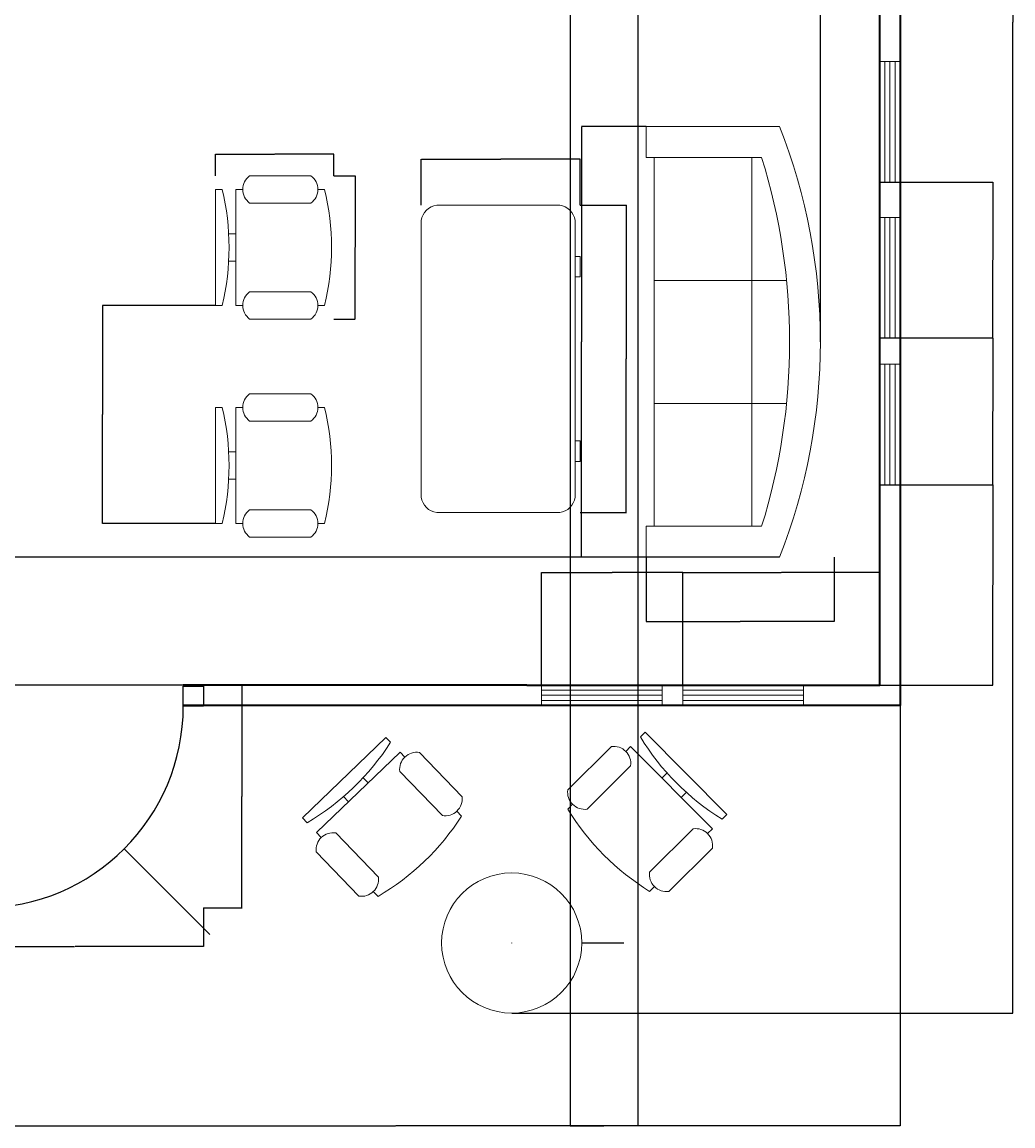
# Model space of a CAD drawing. Units: millimetres. Extents: x 1312 to 12932, y -881 to 10062.
# Tile 3 of 4: x 8020 to 12932, y -881 to 4591. Entities that reach past the tile are written whole.
import ezdxf

# ---------------------------------------------------------------- set-up
doc = ezdxf.new("R2010")
doc.units = ezdxf.units.MM
for name, color, linetype, lineweight in [('A-ANNO-DIMS', 2, 'Continuous', 18), ('A-DOOR', 3, 'Continuous', 25), ('A-FURN', 8, 'Continuous', 18), ('A-GLAZ', 4, 'Continuous', 18), ('A-WALL', 7, 'Continuous', 35)]:
    doc.layers.add(name, color=color, linetype=linetype, lineweight=lineweight)
doc.styles.get("Standard").update_dxf_attribs({"font": 'arial.ttf'})
doc.dimstyles.get("Standard").update_dxf_attribs({"dimtxt": 0.18, "dimasz": 0.18, "dimexe": 0.18, "dimexo": 0.0625, "dimgap": 0.09, "dimtad": 0, "dimtih": 1, "dimtoh": 1, "dimdec": 4, "dimzin": 0, "dimdsep": 46, "dimtxsty": 'Standard', "dimcen": 0.09, "dimadec": 0, "dimazin": 0, "dimtfac": 1, "dimtdec": 4, "dimtofl": 0, "dimtmove": 0, "dimatfit": 3, "dimfxl": 1, "dimtolj": 1, "dimtzin": 0, "dimarcsym": 0})

# ---------------------------------------------------------------- blocks, each defined once
blk = doc.blocks.new('Sofa - Roundback 7 ft.')
for p, q in [((-12.00002, -32.4421), (-12.00003, -6.5971)), ((11.99997, -32.4421), (11.99998, -6.5971)), ((-36.000027, -34), (-36.000027, -11.4696)), ((35.99998, -34), (35.99998, -11.4696)), ((-35.999844, -13.3819), (35.9998, -13.3819)), ((-36.000027, -32.4421), (35.99998, -32.4421))]:
    blk.add_line(p, q)
for points in [[(-36.000027, -34), (-42.000027, -34), (-42.000027, -8)], [(41.99998, -8), (41.99998, -34), (35.99998, -34)]]:
    blk.add_lwpolyline(points)
for centre, radius, start, end in [((0, -114.25), 114.25, 68.43141, 111.5686), ((-0.00001, -127.1968), 121.1968, 72.72033, 107.2797)]:
    blk.add_arc(centre, radius, start, end)
blk = doc.blocks.new('Chair - Desk')
for p, q in [((-8.5, 0), (-8.5, -1)), ((-8.5, 0), (8.5, 0)), ((8.5, 0), (8.5, -1)), ((-8.5, -3), (-8.5, -4)), ((-8.5, -3), (8.5, -3)), ((-2, -3), (-2, -1.9355)), ((2, -1.9576), (2, -3)), ((8.5, -3), (8.5, -4)), ((-10.5, -5), (-10.5, -14)), ((-6.5, -14), (-6.5, -5)), ((6.5, -5), (6.5, -14)), ((10.5, -14), (10.5, -5)), ((-8.5, -15), (-8.5, -16)), ((8.5, -15), (8.5, -16))]:
    blk.add_line(p, q)
for centre, radius, start, end in [((0, 34.625), 36.625, 256.5803, 283.4197), ((-8.5, -6.5), 2.5, 36.8699, 143.1301), ((8.5, -6.5), 2.5, 36.8699, 143.1301), ((-8.5, -12.5), 2.5, 216.8699, 323.1301), ((8.5, -12.5), 2.5, 216.8699, 323.1301), ((0, 19.625), 36.625, 256.5803, 283.4197)]:
    blk.add_arc(centre, radius, start, end)
blk = doc.blocks.new('Desk - 30 x 60 in.')
for p, q in [((-26.999995, 0), (26.999995, 0)), ((-29.999995, -27), (-29.999995, -3)), ((29.999995, -3), (29.999995, -27)), ((26.999995, -30), (-26.999995, -30)), ((-20.000005, -30), (-20.000005, -31)), ((-16.000005, -31), (-16.000005, -30)), ((15.999995, -31), (15.999995, -30)), ((19.999995, -30), (19.999995, -31)), ((-20.000005, -31), (-16.000005, -31)), ((19.999995, -31), (15.999995, -31))]:
    blk.add_line(p, q)
for centre, start, end in [((-26.499995, -3.5), 98.1301, 171.8699), ((26.499995, -3.5), 8.130102, 81.8699), ((-26.499995, -26.5), 188.1301, 261.8699), ((26.499995, -26.5), 278.1301, 351.8699)]:
    blk.add_arc(centre, 3.535534, start, end)
blk = doc.blocks.new('Window - Wood Frame 36 in. Wide plan')
for p, q in [((0, 6), (0, 0)), ((0, 4.5), (36, 4.5)), ((36, 6), (36, 0)), ((0, 3), (36, 3)), ((0, 1.5), (36, 1.5))]:
    blk.add_line(p, q)
blk = doc.blocks.new('DOOR-SINGLE-1000')
for p, q in [((0, 1003.8), (0, 1103.8)), ((0, 1103.8), (100, 1103.8)), ((100, 1103.8), (100, 1003.8)), ((1174.2, 1000), (1174.2, 1100)), ((1174.2, 1100), (1274.2, 1100)), ((1274.2, 1100), (1274.2, 1000)), ((100, 1003.8), (0, 1003.8)), ((100, 1000), (174.2, 1000)), ((100, 0), (100, 1000)), ((174.2, 1000), (174.2, 0)), ((1274.2, 1000), (1174.2, 1000)), ((174.2, 0), (100, 0))]:
    blk.add_line(p, q)
blk.add_arc((174.2, 1000), 1000, 270, 0)
blk = doc.blocks.new('*D15')
at = {"layer": 'A-ANNO-DIMS', "color": 0, "lineweight": -2, "transparency": 16777216}
for p, q in [((7644.9, 199.3), (7644.9, 8)), ((8919.1, 199.3), (8919.1, 8)), ((7645.1, 8.2), (8280.6, 8.2)), ((8918.9, 8.2), (8283.4, 8.2))]:
    blk.add_line(p, q, dxfattribs=at)
at = {"layer": 'A-ANNO-DIMS', "color": 0, "transparency": 16777216}
for points in [[(7645.1, 8.2), (7645.1, 8.2), (7644.9, 8.2)], [(8918.9, 8.2), (8918.9, 8.2), (8919.1, 8.2)]]:
    blk.add_solid(points, dxfattribs=at)
at = {"layer": 'Defpoints', "color": 0, "transparency": 16777216}
for p in [(7644.9, 199.3), (8919.1, 199.3), (8919.1, 8.2)]:
    blk.add_point(p, dxfattribs=at)
at = {"layer": 'A-ANNO-DIMS', "color": 0, "transparency": 16777216, "insert": (8282, 8.2), "char_height": 0.18, "attachment_point": 5}
blk.add_mtext('\\A1;DOOR UNIT 1274 TYP.', dxfattribs=at)
blk = doc.blocks.new('*D16')
at = {"layer": 'A-ANNO-DIMS', "color": 0, "lineweight": -2, "transparency": 16777216}
for p, q in [((8919.2, 1303.1), (9110.4, 1303.1)), ((9110.2, 1302.9), (9110.2, 751.4)), ((9110.2, 199.5), (9110.2, 751)), ((8919.2, 199.3), (9110.4, 199.3))]:
    blk.add_line(p, q, dxfattribs=at)
at = {"layer": 'A-ANNO-DIMS', "color": 0, "transparency": 16777216}
for points in [[(9110.2, 1302.9), (9110.3, 1302.9), (9110.2, 1303.1)], [(9110.2, 199.5), (9110.3, 199.5), (9110.2, 199.3)]]:
    blk.add_solid(points, dxfattribs=at)
at = {"layer": 'Defpoints', "color": 0, "transparency": 16777216}
for p in [(8919.1, 1303.1), (9110.2, 1303.1), (8919.1, 199.3)]:
    blk.add_point(p, dxfattribs=at)
at = {"layer": 'A-ANNO-DIMS', "color": 0, "transparency": 16777216, "insert": (9110.2, 751.2), "char_height": 0.18, "attachment_point": 5}
blk.add_mtext('\\A1;1104 TYP.', dxfattribs=at)
blk = doc.blocks.new('*D17')
at = {"layer": 'A-ANNO-DIMS', "color": 0, "lineweight": -2, "transparency": 16777216}
for p, q in [((9564.9, 3829), (9671.6, 3829)), ((9671.4, 3828.8), (9671.4, 3474)), ((9671.4, 3118.8), (9671.4, 3473.6)), ((9564.9, 3118.7), (9671.6, 3118.7))]:
    blk.add_line(p, q, dxfattribs=at)
at = {"layer": 'A-ANNO-DIMS', "color": 0, "transparency": 16777216}
for points in [[(9671.4, 3828.8), (9671.4, 3828.8), (9671.4, 3829)], [(9671.4, 3118.8), (9671.4, 3118.8), (9671.4, 3118.7)]]:
    blk.add_solid(points, dxfattribs=at)
at = {"layer": 'Defpoints', "color": 0, "transparency": 16777216}
for p in [(9564.9, 3829), (9671.4, 3829), (9564.9, 3118.7)]:
    blk.add_point(p, dxfattribs=at)
at = {"layer": 'A-ANNO-DIMS', "color": 0, "transparency": 16777216, "insert": (9671.4, 3473.8), "char_height": 0.18, "attachment_point": 5}
blk.add_mtext('\\A1;CHAIR 710 TYP.', dxfattribs=at)
blk = doc.blocks.new('*D18')
at = {"layer": 'A-ANNO-DIMS', "color": 0, "lineweight": -2, "transparency": 16777216}
for p, q in [((8978.6, 3829), (8978.6, 3935.7)), ((8978.8, 3935.5), (9271.1, 3935.5)), ((9564.7, 3935.5), (9272.3, 3935.5)), ((9564.9, 3829), (9564.9, 3935.7))]:
    blk.add_line(p, q, dxfattribs=at)
at = {"layer": 'A-ANNO-DIMS', "color": 0, "transparency": 16777216}
for points in [[(8978.8, 3935.5), (8978.8, 3935.5), (8978.6, 3935.5)], [(9564.7, 3935.5), (9564.7, 3935.5), (9564.9, 3935.5)]]:
    blk.add_solid(points, dxfattribs=at)
at = {"layer": 'Defpoints', "color": 0, "transparency": 16777216}
for p in [(8978.6, 3935.5), (8978.6, 3829), (9564.9, 3829)]:
    blk.add_point(p, dxfattribs=at)
at = {"layer": 'A-ANNO-DIMS', "color": 0, "transparency": 16777216, "insert": (9271.7, 3935.5), "char_height": 0.18, "attachment_point": 5}
blk.add_mtext('\\A1;586 TYP.', dxfattribs=at)
blk = doc.blocks.new('*D37')
at = {"layer": 'A-ANNO-DIMS', "color": 0, "lineweight": -2, "transparency": 16777216}
for p, q in [((11113.5, 4072.2), (10793.4, 4072.2)), ((10793.6, 4072), (10793.6, 3005.6)), ((10793.6, 1938.8), (10793.6, 3005.2)), ((11113.5, 1938.6), (10793.4, 1938.6))]:
    blk.add_line(p, q, dxfattribs=at)
at = {"layer": 'A-ANNO-DIMS', "color": 0, "transparency": 16777216}
for points in [[(10793.5, 4072), (10793.6, 4072), (10793.6, 4072.2)], [(10793.5, 1938.8), (10793.6, 1938.8), (10793.6, 1938.6)]]:
    blk.add_solid(points, dxfattribs=at)
at = {"layer": 'Defpoints', "color": 0, "transparency": 16777216}
for p in [(11113.6, 4072.2), (10793.6, 1938.6), (11113.6, 1938.6)]:
    blk.add_point(p, dxfattribs=at)
at = {"layer": 'A-ANNO-DIMS', "color": 0, "transparency": 16777216, "insert": (10793.6, 3005.4), "char_height": 0.18, "attachment_point": 5}
blk.add_mtext('\\A1;SOFA 2134', dxfattribs=at)
blk = doc.blocks.new('*D38')
at = {"layer": 'A-ANNO-DIMS', "color": 0, "lineweight": -2, "transparency": 16777216}
for p, q in [((11113.6, 1938.5), (11113.6, 1618.4)), ((12044.9, 1938.5), (12044.9, 1618.4)), ((11113.8, 1618.6), (11579, 1618.6)), ((12044.8, 1618.6), (11579.6, 1618.6))]:
    blk.add_line(p, q, dxfattribs=at)
at = {"layer": 'A-ANNO-DIMS', "color": 0, "transparency": 16777216}
for points in [[(11113.8, 1618.6), (11113.8, 1618.5), (11113.6, 1618.6)], [(12044.8, 1618.6), (12044.8, 1618.5), (12044.9, 1618.6)]]:
    blk.add_solid(points, dxfattribs=at)
at = {"layer": 'Defpoints', "color": 0, "transparency": 16777216}
for p in [(11113.6, 1938.6), (12044.9, 1938.6), (12044.9, 1618.6)]:
    blk.add_point(p, dxfattribs=at)
at = {"layer": 'A-ANNO-DIMS', "color": 0, "transparency": 16777216, "insert": (11579.3, 1618.6), "char_height": 0.18, "attachment_point": 5}
blk.add_mtext('\\A1;931', dxfattribs=at)
blk = doc.blocks.new('*D39')
at = {"layer": 'A-ANNO-DIMS', "color": 0, "lineweight": -2, "transparency": 16777216}
for p, q in [((10786.6, 3683), (11015.3, 3683)), ((11015.1, 3682.9), (11015.1, 2921.2)), ((11015.1, 2159.2), (11015.1, 2920.9)), ((10786.6, 2159), (11015.3, 2159))]:
    blk.add_line(p, q, dxfattribs=at)
at = {"layer": 'A-ANNO-DIMS', "color": 0, "transparency": 16777216}
for points in [[(11015.1, 3682.9), (11015.1, 3682.9), (11015.1, 3683)], [(11015.1, 2159.2), (11015.1, 2159.2), (11015.1, 2159)]]:
    blk.add_solid(points, dxfattribs=at)
at = {"layer": 'Defpoints', "color": 0, "transparency": 16777216}
for p in [(10786.5, 3683), (11015.1, 3683), (10786.5, 2159)]:
    blk.add_point(p, dxfattribs=at)
at = {"layer": 'A-ANNO-DIMS', "color": 0, "transparency": 16777216, "insert": (11015.1, 2921), "char_height": 0.18, "attachment_point": 5}
blk.add_mtext('\\A1;DESK 1524', dxfattribs=at)
blk = doc.blocks.new('*D40')
at = {"layer": 'A-ANNO-DIMS', "color": 0, "lineweight": -2, "transparency": 16777216}
for p, q in [((9999.1, 3683.1), (9999.1, 3911.8)), ((9999.3, 3911.6), (10392.5, 3911.6)), ((10786.3, 3911.6), (10393.1, 3911.6)), ((10786.5, 3683.1), (10786.5, 3911.8))]:
    blk.add_line(p, q, dxfattribs=at)
at = {"layer": 'A-ANNO-DIMS', "color": 0, "transparency": 16777216}
for points in [[(9999.3, 3911.7), (9999.3, 3911.6), (9999.1, 3911.6)], [(10786.3, 3911.7), (10786.3, 3911.6), (10786.5, 3911.6)]]:
    blk.add_solid(points, dxfattribs=at)
at = {"layer": 'Defpoints', "color": 0, "transparency": 16777216}
for p in [(9999.1, 3911.6), (9999.1, 3683), (10786.5, 3683)]:
    blk.add_point(p, dxfattribs=at)
at = {"layer": 'A-ANNO-DIMS', "color": 0, "transparency": 16777216, "insert": (10392.8, 3911.6), "char_height": 0.18, "attachment_point": 5}
blk.add_mtext('\\A1;787', dxfattribs=at)
blk = doc.blocks.new('*D59')
at = {"layer": 'A-ANNO-DIMS', "color": 0, "lineweight": -2, "transparency": 16777216}
for p, q in [((7372, 1203), (7372, -881.3)), ((12372, 1203), (12372, -881.3)), ((7372.2, -881.1), (9871.6, -881.1)), ((12371.8, -881.1), (9872.4, -881.1))]:
    blk.add_line(p, q, dxfattribs=at)
at = {"layer": 'A-ANNO-DIMS', "color": 0, "transparency": 16777216}
for points in [[(7372.2, -881), (7372.2, -881.1), (7372, -881.1)], [(12371.8, -881), (12371.8, -881.1), (12372, -881.1)]]:
    blk.add_solid(points, dxfattribs=at)
at = {"layer": 'Defpoints', "color": 0, "transparency": 16777216}
for p in [(7372, 1203.1), (12372, 1203.1), (12372, -881.1)]:
    blk.add_point(p, dxfattribs=at)
at = {"layer": 'A-ANNO-DIMS', "color": 0, "transparency": 16777216, "insert": (9872, -881.1), "char_height": 0.18, "attachment_point": 5}
blk.add_mtext('\\A1;5000', dxfattribs=at)
blk = doc.blocks.new('*D72')
at = {"layer": 'A-ANNO-DIMS', "color": 0, "lineweight": -2, "transparency": 16777216}
for p, q in [((10594.2, 1303.2), (10594.2, 1862.5)), ((10594.4, 1862.3), (10944.4, 1862.3)), ((11295.1, 1862.3), (10945.1, 1862.3)), ((11295.3, 1303.2), (11295.3, 1862.5))]:
    blk.add_line(p, q, dxfattribs=at)
at = {"layer": 'A-ANNO-DIMS', "color": 0, "transparency": 16777216}
for points in [[(10594.4, 1862.4), (10594.4, 1862.3), (10594.2, 1862.3)], [(11295.1, 1862.4), (11295.1, 1862.3), (11295.3, 1862.3)]]:
    blk.add_solid(points, dxfattribs=at)
at = {"layer": 'Defpoints', "color": 0, "transparency": 16777216}
for p in [(11295.3, 1862.3), (10594.2, 1303.1), (11295.3, 1303.1)]:
    blk.add_point(p, dxfattribs=at)
at = {"layer": 'A-ANNO-DIMS', "color": 0, "transparency": 16777216, "insert": (10944.8, 1862.3), "char_height": 0.18, "attachment_point": 5}
blk.add_mtext('\\A1;701.1', dxfattribs=at)
blk = doc.blocks.new('*D73')
at = {"layer": 'A-ANNO-DIMS', "color": 0, "lineweight": -2, "transparency": 16777216}
for p, q in [((11295.3, 1303.2), (11295.3, 1862.5)), ((11295.5, 1862.3), (11783.3, 1862.3)), ((12271.8, 1862.3), (11784, 1862.3)), ((12272, 1303.2), (12272, 1862.5))]:
    blk.add_line(p, q, dxfattribs=at)
at = {"layer": 'A-ANNO-DIMS', "color": 0, "transparency": 16777216}
for points in [[(11295.5, 1862.4), (11295.5, 1862.3), (11295.3, 1862.3)], [(12271.8, 1862.4), (12271.8, 1862.3), (12272, 1862.3)]]:
    blk.add_solid(points, dxfattribs=at)
at = {"layer": 'Defpoints', "color": 0, "transparency": 16777216}
for p in [(12272, 1862.3), (11295.3, 1303.1), (12272, 1303.1)]:
    blk.add_point(p, dxfattribs=at)
at = {"layer": 'A-ANNO-DIMS', "color": 0, "transparency": 16777216, "insert": (11783.6, 1862.3), "char_height": 0.18, "attachment_point": 5}
blk.add_mtext('\\A1;976.7', dxfattribs=at)
blk = doc.blocks.new('*D74')
at = {"layer": 'A-ANNO-DIMS', "color": 0, "lineweight": -2, "transparency": 16777216}
for p, q in [((12272.4, 2297.2), (12831.7, 2297.1)), ((12831.6, 2296.9), (12831.4, 1800.2)), ((12831.2, 1303.1), (12831.4, 1799.8)), ((12272.1, 1303.1), (12831.4, 1302.9))]:
    blk.add_line(p, q, dxfattribs=at)
at = {"layer": 'A-ANNO-DIMS', "color": 0, "transparency": 16777216}
for points in [[(12831.5, 2296.9), (12831.6, 2296.9), (12831.6, 2297.1)], [(12831.2, 1303.1), (12831.3, 1303.1), (12831.2, 1302.9)]]:
    blk.add_solid(points, dxfattribs=at)
at = {"layer": 'Defpoints', "color": 0, "transparency": 16777216}
for p in [(12272.3, 2297.2), (12272, 1303.1), (12831.2, 1302.9)]:
    blk.add_point(p, dxfattribs=at)
at = {"layer": 'A-ANNO-DIMS', "color": 0, "transparency": 16777216, "insert": (12831.4, 1800), "char_height": 0.18, "attachment_point": 5}
blk.add_mtext('\\A1;994.1', dxfattribs=at)
blk = doc.blocks.new('*D75')
at = {"layer": 'A-ANNO-DIMS', "color": 0, "lineweight": -2, "transparency": 16777216}
for p, q in [((12272.4, 3024.6), (12831.7, 3024.6)), ((12831.6, 3024.4), (12831.6, 2661.1)), ((12831.6, 2297.4), (12831.6, 2660.7)), ((12272.4, 2297.2), (12831.7, 2297.2))]:
    blk.add_line(p, q, dxfattribs=at)
at = {"layer": 'A-ANNO-DIMS', "color": 0, "transparency": 16777216}
for points in [[(12831.5, 3024.4), (12831.6, 3024.4), (12831.6, 3024.6)], [(12831.5, 2297.4), (12831.6, 2297.4), (12831.6, 2297.2)]]:
    blk.add_solid(points, dxfattribs=at)
at = {"layer": 'Defpoints', "color": 0, "transparency": 16777216}
for p in [(12272.3, 3024.6), (12272.3, 2297.2), (12831.6, 2297.2)]:
    blk.add_point(p, dxfattribs=at)
at = {"layer": 'A-ANNO-DIMS', "color": 0, "transparency": 16777216, "insert": (12831.6, 2660.9), "char_height": 0.18, "attachment_point": 5}
blk.add_mtext('\\A1;727.4', dxfattribs=at)
blk = doc.blocks.new('*D76')
at = {"layer": 'A-ANNO-DIMS', "color": 0, "lineweight": -2, "transparency": 16777216}
for p, q in [((12272.4, 3797.7), (12831.7, 3797.7)), ((12831.6, 3797.5), (12831.6, 3411.3)), ((12831.6, 3024.8), (12831.6, 3411)), ((12272.4, 3024.6), (12831.7, 3024.6))]:
    blk.add_line(p, q, dxfattribs=at)
at = {"layer": 'A-ANNO-DIMS', "color": 0, "transparency": 16777216}
for points in [[(12831.5, 3797.5), (12831.6, 3797.5), (12831.6, 3797.7)], [(12831.5, 3024.8), (12831.6, 3024.8), (12831.6, 3024.6)]]:
    blk.add_solid(points, dxfattribs=at)
at = {"layer": 'Defpoints', "color": 0, "transparency": 16777216}
for p in [(12272.3, 3797.7), (12272.3, 3024.6), (12831.6, 3024.6)]:
    blk.add_point(p, dxfattribs=at)
at = {"layer": 'A-ANNO-DIMS', "color": 0, "transparency": 16777216, "insert": (12831.6, 3411.1), "char_height": 0.18, "attachment_point": 5}
blk.add_mtext('\\A1;773', dxfattribs=at)
blk = doc.blocks.new('*D81')
at = {"layer": 'A-ANNO-DIMS', "color": 0, "lineweight": -2, "transparency": 16777216}
for p, q in [((12372.1, 9503.1), (12931.4, 9503.1)), ((12931.2, 9502.9), (12931.2, 4590.8)), ((12931.2, -321.6), (12931.2, 4590.4)), ((10447.2, -321.8), (12931.4, -321.8))]:
    blk.add_line(p, q, dxfattribs=at)
at = {"layer": 'A-ANNO-DIMS', "color": 0, "transparency": 16777216}
for points in [[(12931.2, 9502.9), (12931.3, 9502.9), (12931.2, 9503.1)], [(12931.2, -321.6), (12931.3, -321.6), (12931.2, -321.8)]]:
    blk.add_solid(points, dxfattribs=at)
at = {"layer": 'Defpoints', "color": 0, "transparency": 16777216}
for p in [(12372, 9503.1), (12931.2, 9503.1), (10447.2, -321.8)]:
    blk.add_point(p, dxfattribs=at)
at = {"layer": 'A-ANNO-DIMS', "color": 0, "transparency": 16777216, "insert": (12931.2, 4590.6), "char_height": 0.18, "attachment_point": 5}
blk.add_mtext('\\A1;9825', dxfattribs=at)
blk = doc.blocks.new('*D90')
at = {"layer": 'A-ANNO-DIMS', "color": 0, "lineweight": -2, "transparency": 16777216}
for p, q in [((10737.2, 9364.9), (10737.2, -881.3)), ((11072, 9403), (11072, -881.3)), ((10737.4, -881.1), (10904.2, -881.1)), ((11071.8, -881.1), (10905, -881.1))]:
    blk.add_line(p, q, dxfattribs=at)
at = {"layer": 'A-ANNO-DIMS', "color": 0, "transparency": 16777216}
for points in [[(10737.4, -881), (10737.4, -881.1), (10737.2, -881.1)], [(11071.8, -881), (11071.8, -881.1), (11072, -881.1)]]:
    blk.add_solid(points, dxfattribs=at)
at = {"layer": 'Defpoints', "color": 0, "transparency": 16777216}
for p in [(10737.2, 9365), (11072, 9403.1), (11072, -881.1)]:
    blk.add_point(p, dxfattribs=at)
at = {"layer": 'A-ANNO-DIMS', "color": 0, "transparency": 16777216, "insert": (10904.6, -881.1), "char_height": 0.18, "attachment_point": 5}
blk.add_mtext('\\A1;334.8', dxfattribs=at)
blk = doc.blocks.new('*D95')
at = {"layer": 'A-ANNO-DIMS', "color": 0, "lineweight": -2, "transparency": 16777216}
for p, q in [((11977.2, 3005.5), (11977.2, 10062.5)), ((11977.4, 10062.3), (12124.4, 10062.3)), ((12272.1, 10062.3), (12125.1, 10062.3)), ((12272.3, 3024.7), (12272.3, 10062.5))]:
    blk.add_line(p, q, dxfattribs=at)
at = {"layer": 'A-ANNO-DIMS', "color": 0, "transparency": 16777216}
for points in [[(11977.4, 10062.3), (11977.4, 10062.3), (11977.2, 10062.3)], [(12272.1, 10062.3), (12272.1, 10062.3), (12272.3, 10062.3)]]:
    blk.add_solid(points, dxfattribs=at)
at = {"layer": 'Defpoints', "color": 0, "transparency": 16777216}
for p in [(12272.3, 10062.3), (12272.3, 3024.6), (11977.2, 3005.4)]:
    blk.add_point(p, dxfattribs=at)
at = {"layer": 'A-ANNO-DIMS', "color": 0, "transparency": 16777216, "insert": (12124.8, 10062.3), "char_height": 0.18, "attachment_point": 5}
blk.add_mtext('\\A1;295.1', dxfattribs=at)
blk = doc.blocks.new('*D96')
at = {"layer": 'A-ANNO-DIMS', "color": 0, "lineweight": -2, "transparency": 16777216}
for p, q in [((11773.9, 1938.6), (1312.6, 1938.6)), ((1312.7, 1938.4), (1312.7, 1621)), ((1312.7, 1303.3), (1312.7, 1620.7)), ((12271.9, 1303.1), (1312.6, 1303.1))]:
    blk.add_line(p, q, dxfattribs=at)
at = {"layer": 'A-ANNO-DIMS', "color": 0, "transparency": 16777216}
for points in [[(1312.7, 1938.4), (1312.8, 1938.4), (1312.7, 1938.6)], [(1312.7, 1303.3), (1312.8, 1303.3), (1312.7, 1303.1)]]:
    blk.add_solid(points, dxfattribs=at)
at = {"layer": 'Defpoints', "color": 0, "transparency": 16777216}
for p in [(11774, 1938.6), (1312.7, 1303.1), (12272, 1303.1)]:
    blk.add_point(p, dxfattribs=at)
at = {"layer": 'A-ANNO-DIMS', "color": 0, "transparency": 16777216, "insert": (1312.7, 1620.8), "char_height": 0.18, "attachment_point": 5}
blk.add_mtext('\\A1;635.5', dxfattribs=at)
blk = doc.blocks.new('*D97')
at = {"layer": 'A-ANNO-DIMS', "color": 0, "lineweight": -2, "transparency": 16777216}
for p, q in [((8978.5, 3186.3), (8419.2, 3186.3)), ((8419.3, 3186.1), (8419.3, 2646.1)), ((8419.3, 2105.6), (8419.3, 2645.7)), ((8978.5, 2105.4), (8419.2, 2105.4))]:
    blk.add_line(p, q, dxfattribs=at)
at = {"layer": 'A-ANNO-DIMS', "color": 0, "transparency": 16777216}
for points in [[(8419.3, 3186.1), (8419.4, 3186.1), (8419.3, 3186.3)], [(8419.3, 2105.6), (8419.4, 2105.6), (8419.3, 2105.4)]]:
    blk.add_solid(points, dxfattribs=at)
at = {"layer": 'Defpoints', "color": 0, "transparency": 16777216}
for p in [(8419.3, 3186.3), (8978.6, 3186.3), (8978.6, 2105.4)]:
    blk.add_point(p, dxfattribs=at)
at = {"layer": 'A-ANNO-DIMS', "color": 0, "transparency": 16777216, "insert": (8419.3, 2645.9), "char_height": 0.18, "attachment_point": 5}
blk.add_mtext('\\A1;1080.9', dxfattribs=at)
blk = doc.blocks.new('*D98')
at = {"layer": 'A-ANNO-DIMS', "color": 0, "lineweight": -2, "transparency": 16777216}
for p, q in [((7819, 1199.3), (7819.2, 1199.3)), ((7819.1, 1199.2), (7819.1, 1199.4)), ((8950.5, 67.9), (8526.3, 492.1)), ((8950.6, 67.9), (8950.5, 67.9))]:
    blk.add_line(p, q, dxfattribs=at)
at = {"layer": 'A-ANNO-DIMS', "color": 0, "transparency": 16777216}
blk.add_solid([(8526.4, 492.1), (8526.3, 492.1), (8526.2, 492.2)], dxfattribs=at)
at = {"layer": 'Defpoints', "color": 0, "transparency": 16777216}
for p in [(7819.1, 1199.3), (8526.2, 492.2)]:
    blk.add_point(p, dxfattribs=at)
at = {"layer": 'A-ANNO-DIMS', "color": 0, "transparency": 16777216, "insert": (8951.3, 67.9), "char_height": 0.18, "attachment_point": 5}
blk.add_mtext('\\A1;6X R1000', dxfattribs=at)
blk = doc.blocks.new('*D99')
at = {"layer": 'A-ANNO-DIMS', "color": 0, "lineweight": -2, "transparency": 16777216}
for p, q in [((10447.1, 25.5), (10447.2, 25.5)), ((10447.2, 25.5), (10447.2, 25.6)), ((11003, 25.5), (10794.7, 25.5))]:
    blk.add_line(p, q, dxfattribs=at)
at = {"layer": 'A-ANNO-DIMS', "color": 0, "transparency": 16777216}
blk.add_solid([(10794.7, 25.6), (10794.7, 25.5), (10794.5, 25.5)], dxfattribs=at)
at = {"layer": 'Defpoints', "color": 0, "transparency": 16777216}
for p in [(10099.8, 25.5), (10794.5, 25.5)]:
    blk.add_point(p, dxfattribs=at)
at = {"layer": 'A-ANNO-DIMS', "color": 0, "transparency": 16777216, "insert": (11003.5, 25.5), "char_height": 0.18, "attachment_point": 5}
blk.add_mtext('\\A1;∅694.8', dxfattribs=at)

msp = doc.modelspace()

# ---------------------------------------------------------------- linework, layer by layer
at = {"layer": 'A-FURN'}
msp.add_circle((10447.155, 25.549), 347.378, dxfattribs=at)
at = {"layer": 'A-WALL'}
for p, q in [((12371.992, 9403.061), (12371.992, 1203.088)), ((12271.992, 1303.088), (12271.992, 6703.088)), ((12371.992, 6703.088), (12371.992, 1203.088)), ((10521.992, 1303.088), (8819.096, 1303.088)), ((10521.992, 1303.088), (12271.992, 1303.088)), ((12371.992, 1203.088), (8819.096, 1203.088)), ((10521.992, 1203.088), (8819.096, 1203.088))]:
    msp.add_line(p, q, dxfattribs=at)

# ---------------------------------------------------------------- block references
at = {"layer": 'A-DOOR'}
msp.add_blockref('DOOR-SINGLE-1000', (7644.896, 199.32), dxfattribs=at)
at = {"layer": 'A-FURN'}
for name, p, xscale, yscale, zscale, rotation in [('Sofa - Roundback 7 ft.', (11977.212, 3005.394), 25.4, 25.4, 25.4, 270), ('Chair - Desk', (8978.587, 3473.809), 33.82412471619898, 33.82412471619898, 33.82412471619898, 90), ('Desk - 30 x 60 in.', (9999.104, 2921.046), 25.4, 25.4, 25.4, 90), ('Chair - Desk', (8978.587, 2392.953), 33.82412471619898, 33.82412471619898, 33.82412471619898, 90), ('Chair - Desk', (11311.433, 866.918), 33.82412471619897, 33.82412471619897, 33.82412471619897, 314.8512117112756), ('Chair - Desk', (9616.461, 845.49), 33.82412471619897, 33.82412471619897, 33.82412471619897, 43.90473393060543)]:
    msp.add_blockref(name, p, dxfattribs=dict(at, xscale=xscale, yscale=yscale, zscale=zscale, rotation=rotation))
at = {"layer": 'A-GLAZ', "xscale": 16.61312414671267, "yscale": 16.61312414671267, "zscale": 16.61312414671267, "rotation": 270}
for p in [(12272.313, 4395.758), (12272.313, 3622.681), (12272.313, 2895.303)]:
    msp.add_blockref('Window - Wood Frame 36 in. Wide plan', p, dxfattribs=at)
at = {"layer": 'A-GLAZ', "xscale": 16.61312414671267, "yscale": 16.61312414671267, "zscale": 16.61312414671267}
for p in [(10594.206, 1203.41), (11295.307, 1203.41)]:
    msp.add_blockref('Window - Wood Frame 36 in. Wide plan', p, dxfattribs=at)

# ---------------------------------------------------------------- dimensions: what is measured, and where the dimension line sits
at = {"layer": 'A-ANNO-DIMS'}
for base, p1, p2, override, picture, middle in [((12272.313, 10062.311), (11977.212, 3005.394), (12272.313, 3024.608), {"dimdec": 1, "dimlfac": 1, "dimrnd": 0, "dimzin": 0, "dimdsep": 46, "dimlunit": 2}, '*D95', (12124.763, 10062.311)), ((11071.992, -881.079), (10737.214, 9364.961), (11071.992, 9403.061), {"dimdec": 1, "dimlfac": 1, "dimrnd": 0, "dimzin": 0, "dimdsep": 46, "dimlunit": 2}, '*D90', (10904.603, -881.079)), ((12044.946, 1618.554), (11113.612, 1938.594), (12044.946, 1938.594), {"dimdec": 0, "dimlfac": 1, "dimrnd": 0, "dimzin": 0, "dimdsep": 46, "dimlunit": 2}, '*D38', (11579.279, 1618.554)), ((11295.307, 1862.338), (10594.206, 1303.088), (11295.307, 1303.088), {"dimdec": 1, "dimlfac": 1, "dimrnd": 0, "dimzin": 0, "dimdsep": 46, "dimlunit": 2}, '*D72', (10944.756, 1862.338)), ((12271.992, 1862.338), (11295.307, 1303.088), (12271.992, 1303.088), {"dimdec": 1, "dimlfac": 1, "dimrnd": 0, "dimzin": 0, "dimdsep": 46, "dimlunit": 2}, '*D73', (11783.65, 1862.338)), ((12371.992, -881.079), (7371.992, 1203.088), (12371.992, 1203.088), {"dimdec": 0, "dimlfac": 1, "dimrnd": 0, "dimzin": 0, "dimdsep": 46, "dimlunit": 2}, '*D59', (9871.992, -881.079))]:
    dim = msp.add_linear_dim(base=base, p1=p1, p2=p2, dimstyle='Standard', override=override, dxfattribs=at)
    dim.commit()
    dim.dimension.update_dxf_attribs({"geometry": picture, "text_midpoint": middle})
for base, p1, p2, angle, override, picture, middle in [((12931.242, 9503.061), (10447.155, -321.829), (12371.992, 9503.061), 90, {"dimdec": 0, "dimlfac": 1, "dimrnd": 0, "dimzin": 0, "dimdsep": 46, "dimlunit": 2}, '*D81', (12931.242, 4590.616)), ((9999.104, 3911.646), (10786.504, 3683.046), (9999.104, 3683.046), 180, {"dimdec": 0, "dimlfac": 1, "dimrnd": 0, "dimzin": 0, "dimdsep": 46, "dimlunit": 2}, '*D40', (10392.804, 3911.646)), ((12831.563, 3024.608), (12272.313, 3797.685), (12272.313, 3024.608), 270, {"dimdec": 0, "dimlfac": 1, "dimrnd": 0, "dimzin": 0, "dimdsep": 46, "dimlunit": 2}, '*D76', (12831.563, 3411.147)), ((8419.337, 3186.304), (8978.587, 2105.448), (8978.587, 3186.304), 90, {"dimdec": 1, "dimlfac": 1, "dimrnd": 0, "dimzin": 0, "dimdsep": 46, "dimlunit": 2}, '*D97', (8419.337, 2645.876)), ((12831.563, 2297.231), (12272.313, 3024.608), (12272.313, 2297.231), 270, {"dimdec": 1, "dimlfac": 1, "dimrnd": 0, "dimzin": 0, "dimdsep": 46, "dimlunit": 2}, '*D75', (12831.563, 2660.919)), ((12831.242, 1302.908), (12272.313, 2297.231), (12271.992, 1303.088), 269.981485, {"dimdec": 1, "dimlfac": 1, "dimrnd": 0, "dimzin": 0, "dimdsep": 46, "dimlunit": 2}, '*D74', (12831.403, 1799.979)), ((1312.742, 1303.088), (11774.012, 1938.594), (12271.992, 1303.088), 90, {"dimdec": 1, "dimlfac": 1, "dimrnd": 0, "dimzin": 0, "dimdsep": 46, "dimlunit": 2}, '*D96', (1312.742, 1620.841))]:
    dim = msp.add_linear_dim(base=base, p1=p1, p2=p2, angle=angle, dimstyle='Standard', override=override, dxfattribs=at)
    dim.commit()
    dim.dimension.update_dxf_attribs({"geometry": picture, "text_midpoint": middle})
for base, p1, p2, angle, text, picture, middle in [((10793.572, 1938.594), (11113.612, 4072.194), (11113.612, 1938.594), 270, 'SOFA <>', '*D37', (10793.572, 3005.394)), ((8978.587, 3935.509), (9564.872, 3828.963), (8978.587, 3828.963), 180, '<> TYP.', '*D18', (9271.729, 3935.509)), ((9671.418, 3828.963), (9564.872, 3118.656), (9564.872, 3828.963), 90, 'CHAIR <> TYP.', '*D17', (9671.418, 3473.809)), ((11015.104, 3683.046), (10786.504, 2159.046), (10786.504, 3683.046), 90, 'DESK <>', '*D39', (11015.104, 2921.046)), ((9110.226, 1303.088), (8919.096, 199.32), (8919.096, 1303.088), 90, '<> TYP.', '*D16', (9110.226, 751.204))]:
    dim = msp.add_linear_dim(base=base, p1=p1, p2=p2, angle=angle, text=text, dimstyle='Standard', override={"dimdec": 0, "dimlfac": 1, "dimrnd": 0, "dimzin": 0, "dimdsep": 46, "dimlunit": 2}, dxfattribs=at)
    dim.commit()
    dim.dimension.update_dxf_attribs({"geometry": picture, "text_midpoint": middle})
dim = msp.add_radius_dim(center=(7819.096, 1199.32), mpoint=(8526.203, 492.213), text='6X <>', dimstyle='Standard', override={"dimdec": 0, "dimlfac": 1, "dimrnd": 0, "dimzin": 0, "dimdsep": 46, "dimlunit": 2}, dxfattribs=at)
dim.commit()
dim.dimension.update_dxf_attribs({"geometry": '*D98', "text_midpoint": (8951.285, 67.949), "dimtype": 164})
dim = msp.add_linear_dim(base=(8919.096, 8.19), p1=(7644.896, 199.32), p2=(8919.096, 199.32), text='DOOR UNIT <> TYP.', dimstyle='Standard', override={"dimdec": 0, "dimlfac": 1, "dimrnd": 0, "dimzin": 0, "dimdsep": 46, "dimlunit": 2}, dxfattribs=at)
dim.commit()
dim.dimension.update_dxf_attribs({"geometry": '*D15', "text_midpoint": (8281.996, 8.19)})
dim = msp.add_diameter_dim_2p(p1=(10099.777, 25.55), p2=(10794.533, 25.549), dimstyle='Standard', override={"dimdec": 1, "dimlfac": 1, "dimrnd": 0, "dimzin": 0, "dimdsep": 46, "dimlunit": 2}, dxfattribs=at)
dim.commit()
dim.dimension.update_dxf_attribs({"geometry": '*D99', "text_midpoint": (11002.959, 25.549), "dimtype": 163})

doc.saveas('drawing.dxf')
